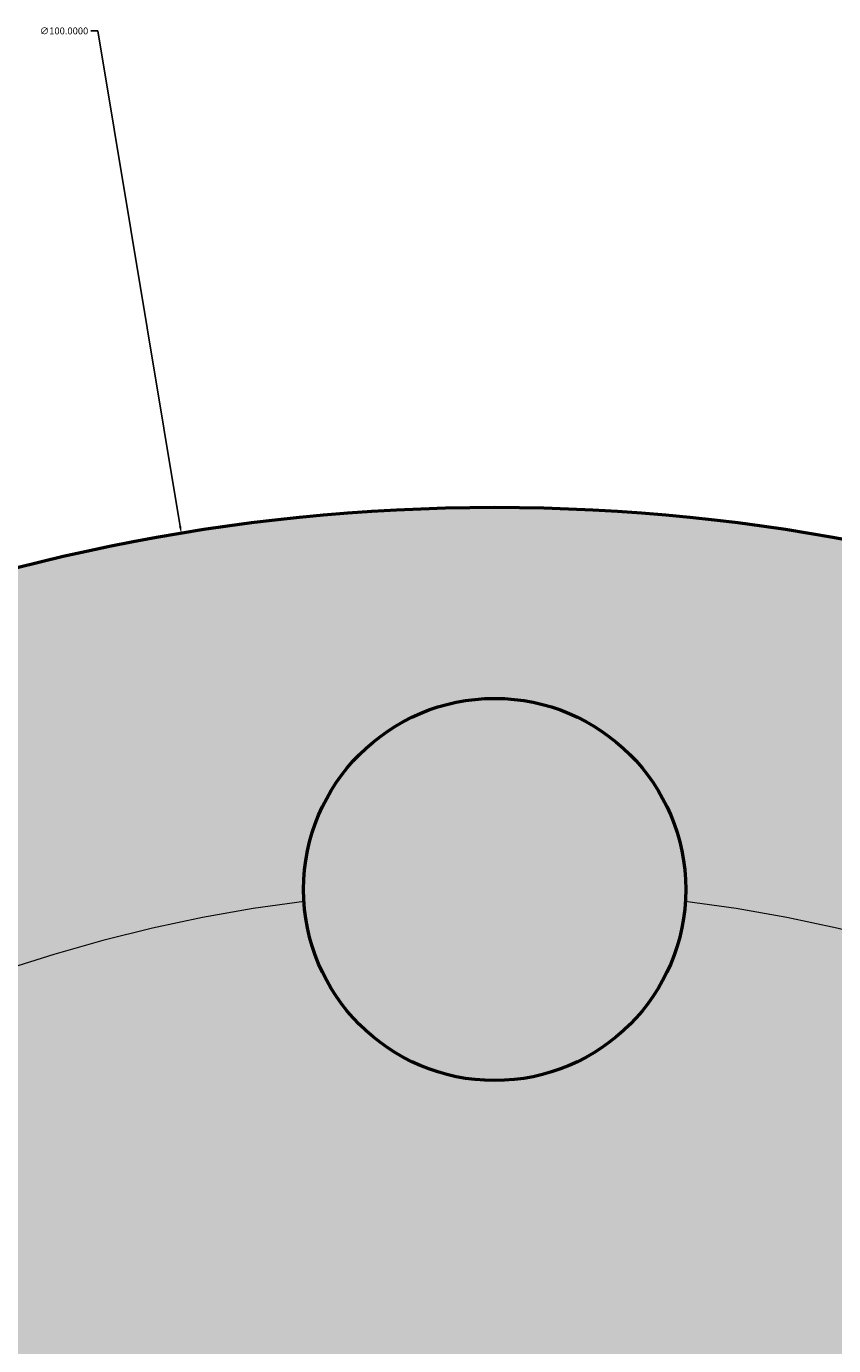
# Model space of a CAD drawing. Units: inches. Extents: x 139261 to 139415, y 52839 to 52963.
# Tile 18 of 20: x 139328 to 139349, y 52928 to 52963. Entities that reach past the tile are written whole.
import ezdxf

# ---------------------------------------------------------------- set-up
doc = ezdxf.new("R2010")
doc.units = ezdxf.units.IN
doc.header["$MEASUREMENT"] = 0
doc.linetypes.add('CENTER', pattern=[50.8, 31.75, -6.35, 6.35, -6.35])
for name, color, linetype, lineweight in [('M-CNTR', 4, 'CENTER', 18), ('M-DIMS', 2, 'Continuous', 25), ('M-HATC', 8, 'Continuous', 18), ('M-OUTL', 7, 'Continuous', 50)]:
    doc.layers.add(name, color=color, linetype=linetype, lineweight=lineweight)
doc.styles.get("Standard").update_dxf_attribs({"font": 'arial.ttf'})
doc.dimstyles.get("Standard").update_dxf_attribs({"dimtxt": 0.18, "dimasz": 0.18, "dimexe": 0.18, "dimexo": 0.0625, "dimgap": 0.09, "dimtad": 0, "dimtih": 1, "dimtoh": 1, "dimdec": 4, "dimzin": 0, "dimdsep": 46, "dimtxsty": 'Standard', "dimcen": 0.09, "dimadec": 0, "dimazin": 0, "dimtfac": 1, "dimtdec": 4, "dimtofl": 0, "dimtmove": 0, "dimatfit": 3, "dimfxl": 1, "dimtolj": 1, "dimtzin": 0, "dimarcsym": 0})

# ---------------------------------------------------------------- blocks, each defined once
blk = doc.blocks.new('*U1')
blk.add_circle((0, 0), 5)
blk = doc.blocks.new('*U2')
at = {"layer": 'M-OUTL', "color": 0, "linetype": 'ByBlock', "lineweight": -2, "transparency": 16777216}
blk.add_blockref('*U1', (139340.357, 52940.217), dxfattribs=at)
blk = doc.blocks.new('*D4')
at = {"layer": 'Defpoints', "color": 0, "transparency": 16777216}
for p in [(139373.053, 52923.26), (139307.661, 52877.175)]:
    blk.add_point(p, dxfattribs=at)
at = {"layer": 'M-DIMS', "color": 0, "lineweight": -2, "transparency": 16777216}
for p, q in [((139414.011, 52952.126), (139373.2, 52923.364)), ((139414.191, 52952.126), (139414.011, 52952.126)), ((139340.267, 52900.217), (139340.447, 52900.217)), ((139340.357, 52900.127), (139340.357, 52900.307))]:
    blk.add_line(p, q, dxfattribs=at)
blk.add_arc((139340.357, 52900.217), 40, 34.9168, 52.0771, dxfattribs=at)
at = {"layer": 'M-DIMS', "color": 0, "transparency": 16777216}
blk.add_solid([(139373.183, 52923.388), (139373.217, 52923.339), (139373.053, 52923.26)], dxfattribs=at)
at = {"layer": 'M-DIMS', "color": 0, "transparency": 16777216, "insert": (139414.822, 52952.126), "char_height": 0.18, "attachment_point": 5}
blk.add_mtext('\\A1;∅80.0000', dxfattribs=at)
blk = doc.blocks.new('*D6')
at = {"layer": 'Defpoints', "color": 0, "transparency": 16777216}
for p in [(139332.153, 52949.54), (139348.561, 52850.895)]:
    blk.add_point(p, dxfattribs=at)
at = {"layer": 'M-DIMS', "color": 0, "lineweight": -2, "transparency": 16777216}
for p, q in [((139329.787, 52962.682), (139329.967, 52962.682)), ((139329.967, 52962.682), (139332.124, 52949.717)), ((139340.267, 52900.217), (139340.447, 52900.217)), ((139340.357, 52900.127), (139340.357, 52900.307))]:
    blk.add_line(p, q, dxfattribs=at)
at = {"layer": 'M-DIMS', "color": 0, "transparency": 16777216}
blk.add_solid([(139332.153, 52949.722), (139332.094, 52949.713), (139332.153, 52949.54)], dxfattribs=at)
at = {"layer": 'M-DIMS', "color": 0, "transparency": 16777216, "insert": (139329.086, 52962.682), "char_height": 0.18, "attachment_point": 5}
blk.add_mtext('\\A1;∅100.0000', dxfattribs=at)
blk = doc.blocks.new('*D9')
at = {"layer": 'Defpoints', "color": 0, "transparency": 16777216}
for p in [(139302.054, 52932.357), (139378.659, 52868.078)]:
    blk.add_point(p, dxfattribs=at)
at = {"layer": 'M-DIMS', "color": 0, "lineweight": -2, "transparency": 16777216}
for p, q in [((139278.893, 52951.64), (139279.073, 52951.64)), ((139279.073, 52951.64), (139301.916, 52932.472)), ((139340.267, 52900.217), (139340.447, 52900.217)), ((139340.357, 52900.127), (139340.357, 52900.307))]:
    blk.add_line(p, q, dxfattribs=at)
at = {"layer": 'M-DIMS', "color": 0, "transparency": 16777216}
blk.add_solid([(139301.936, 52932.495), (139301.897, 52932.449), (139302.054, 52932.357)], dxfattribs=at)
at = {"layer": 'M-DIMS', "color": 0, "transparency": 16777216, "insert": (139278.506, 52951.64), "char_height": 0.18, "attachment_point": 5}
blk.add_mtext('\\A1;∅100', dxfattribs=at)
blk = doc.blocks.new('*D10')
at = {"layer": 'Defpoints', "color": 0, "transparency": 16777216}
for p in [(139325.07, 52937.181), (139355.644, 52863.254)]:
    blk.add_point(p, dxfattribs=at)
at = {"layer": 'M-DIMS', "color": 0, "lineweight": -2, "transparency": 16777216}
for p, q in [((139340.267, 52900.217), (139340.447, 52900.217)), ((139340.357, 52900.127), (139340.357, 52900.307)), ((139364.816, 52841.075), (139355.712, 52863.087)), ((139364.996, 52841.075), (139364.816, 52841.075))]:
    blk.add_line(p, q, dxfattribs=at)
at = {"layer": 'M-DIMS', "color": 0, "transparency": 16777216}
blk.add_solid([(139355.74, 52863.099), (139355.685, 52863.076), (139355.644, 52863.254)], dxfattribs=at)
at = {"layer": 'M-DIMS', "color": 0, "transparency": 16777216, "insert": (139365.312, 52841.075), "char_height": 0.18, "attachment_point": 5}
blk.add_mtext('\\A1;∅80', dxfattribs=at)

msp = doc.modelspace()

# ---------------------------------------------------------------- hatches: boundary and pattern name
at = {"layer": 'M-HATC'}
h = msp.add_hatch(color=256, dxfattribs=at)
h.dxf.hatch_style = 1
h.paths.add_polyline_path([(139290.35689, 52900.21749, 1), (139390.35689, 52900.21749, 1)])
h.paths.add_polyline_path([(139335.36666, 52939.90499, -0.01563646), (139335.35689, 52940.21749, -1), (139345.35689, 52940.21749, -0.01563646), (139345.34711, 52939.90499, -0.13461315), (139364.89157, 52931.80941, -0.691035), (139373.64116, 52928.50176, -0.21521822), (139371.94881, 52924.75216, -0.13461315), (139380.04439, 52905.20771, -0.43265224), (139385.35689, 52900.21749, -0.43265224), (139380.04439, 52895.22726, -0.13461315), (139371.94881, 52875.68281, -0.21521822), (139373.64116, 52871.93321, -0.691035), (139364.89157, 52868.62556, -0.13461315), (139345.34711, 52860.52999, -0.01563646), (139345.35689, 52860.21749, -1), (139335.35689, 52860.21749, -0.01563646), (139335.36666, 52860.52999, -0.13461315), (139315.82221, 52868.62556, -0.691035), (139307.07262, 52871.93321, -0.21521822), (139308.76496, 52875.68281, -0.13461315), (139300.66939, 52895.22726, -0.43265224), (139295.35689, 52900.21749, -0.43265224), (139300.66939, 52905.20771, -0.13461315), (139308.76496, 52924.75216, -0.21521822), (139307.07262, 52928.50176, -0.691035), (139315.82221, 52931.80941, -0.13461315)], flags=16)
h.paths.add_polyline_path([(139365.35689, 52900.21749, -1), (139315.35689, 52900.21749, -1)], flags=0)
h.paths.add_polyline_path([(139323.71474, 52911.30978), (139356.99903, 52911.30978, -0.3027197), (139356.99903, 52889.12519), (139323.71474, 52889.12519, -0.3027197)], flags=0)
h.paths.add_polyline_path([(139364.89157, 52931.80941, 0.13461315), (139345.34711, 52939.90499, -0.93933644), (139335.36666, 52939.90499, 0.13461315), (139315.82221, 52931.80941, -0.18270763), (139317.07262, 52928.50176, -0.64579494), (139308.76496, 52924.75216, 0.13461315), (139300.66939, 52905.20771, -0.39601219), (139305.35689, 52900.21749, -0.39601219), (139300.66939, 52895.22726, 0.13461315), (139308.76496, 52875.68281, -0.64579494), (139317.07262, 52871.93321, -0.18270763), (139315.82221, 52868.62556, 0.13461315), (139335.36666, 52860.52999, -0.93933644), (139345.34711, 52860.52999, 0.13461315), (139364.89157, 52868.62556, -0.18270763), (139363.64116, 52871.93321, -0.64579494), (139371.94881, 52875.68281, 0.13461315), (139380.04439, 52895.22726, -0.39601219), (139375.35689, 52900.21749, -0.39601219), (139380.04439, 52905.20771, 0.13461315), (139371.94881, 52924.75216, -0.64579494), (139363.64116, 52928.50176, -0.18270763)], flags=0)
h = msp.add_hatch(color=256, dxfattribs=at)
h.dxf.hatch_style = 1
h.set_gradient(color1=(205, 105, 40), tint=1)
h.paths.add_polyline_path([(139335.35689, 52940.21749, 1), (139345.35689, 52940.21749, 1)])
h.paths.add_polyline_path([(139307.07262, 52928.50176, 1), (139317.07262, 52928.50176, 1)])
h.paths.add_polyline_path([(139295.35689, 52900.21749, 1), (139305.35689, 52900.21749, 1)])
h.paths.add_polyline_path([(139307.07262, 52871.93321, 1), (139317.07262, 52871.93321, 1)])
h.paths.add_polyline_path([(139345.35689, 52860.21749, 1), (139335.35689, 52860.21749, 1)])
h.paths.add_polyline_path([(139363.64116, 52871.93321, 1), (139373.64116, 52871.93321, 1)])
h.paths.add_polyline_path([(139375.35689, 52900.21749, 1), (139385.35689, 52900.21749, 1)])
h.paths.add_polyline_path([(139363.64116, 52928.50176, 1), (139373.64116, 52928.50176, 1)])
h = msp.add_hatch(color=256, dxfattribs=at)
h.dxf.hatch_style = 1
h.paths.add_polyline_path([(139345.34711, 52939.90499, -0.93933644), (139335.36666, 52939.90499, 0.13461315), (139315.82221, 52931.80941, -0.18270763), (139317.07262, 52928.50176, -0.64579494), (139308.76496, 52924.75216, 0.13461315), (139300.66939, 52905.20771, -0.39601219), (139305.35689, 52900.21749, -0.39601219), (139300.66939, 52895.22726, 0.13461315), (139308.76496, 52875.68281, -0.64579494), (139317.07262, 52871.93321, -0.18270763), (139315.82221, 52868.62556, 0.13461315), (139335.36666, 52860.52999, -0.93933644), (139345.34711, 52860.52999, 0.13461315), (139364.89157, 52868.62556, -0.18270763), (139363.64116, 52871.93321, -0.64579494), (139371.94881, 52875.68281, 0.13461315), (139380.04439, 52895.22726, -0.39601219), (139375.35689, 52900.21749, -0.39601219), (139380.04439, 52905.20771, 0.13461315), (139371.94881, 52924.75216, -0.64579494), (139363.64116, 52928.50176, -0.18270763), (139364.89157, 52931.80941, 0.13461315)])
h.paths.add_polyline_path([(139365.35689, 52900.21749, -1), (139315.35689, 52900.21749, -1)], flags=16)
h.paths.add_polyline_path([(139356.99903, 52911.30978, -0.3027197), (139356.99903, 52889.12519), (139323.71474, 52889.12519, -0.3027197), (139323.71474, 52911.30978)], flags=0)

# ---------------------------------------------------------------- linework, layer by layer
at = {"layer": 'M-CNTR'}
for start, end in [(97.166643, 127.833357), (52.166643, 82.833357)]:
    msp.add_arc((139340.35689, 52900.21749), 40, start, end, dxfattribs=at)
at = {"layer": 'M-OUTL'}
msp.add_circle((139340.35689, 52900.21749), 50, dxfattribs=at)

# ---------------------------------------------------------------- block references
msp.add_blockref('*U2', (0, 0), dxfattribs=at)

# ---------------------------------------------------------------- dimensions: what is measured, and where the dimension line sits
at = {"layer": 'M-DIMS'}
for p1, p2, override, picture, middle in [((139348.56051, 52850.89507), (139332.15326, 52949.5399), {"dimclrd": 0, "dimclre": 0, "dimclrt": 0}, '*D6', (139329.08622, 52962.68242)), ((139307.66087, 52877.17469), (139373.0529, 52923.26028), {"dimclrd": 0, "dimclre": 0, "dimclrt": 0}, '*D4', (139414.82217, 52952.12585)), ((139378.65939, 52868.07845), (139302.05438, 52932.35652), {"dimdec": 0, "dimlfac": 1, "dimrnd": 0, "dimzin": 0, "dimdsep": 46, "dimlunit": 2}, '*D9', (139278.50641, 52951.63995)), ((139325.07023, 52937.18123), (139355.64354, 52863.25374), {"dimdec": 0, "dimlfac": 1, "dimrnd": 0, "dimzin": 0, "dimdsep": 46, "dimlunit": 2}, '*D10', (139365.31206, 52841.0755))]:
    dim = msp.add_diameter_dim_2p(p1=p1, p2=p2, dimstyle='Standard', override=override, dxfattribs=at)
    dim.commit()
    dim.dimension.update_dxf_attribs({"geometry": picture, "text_midpoint": middle, "dimtype": 163})

doc.saveas('drawing.dxf')
